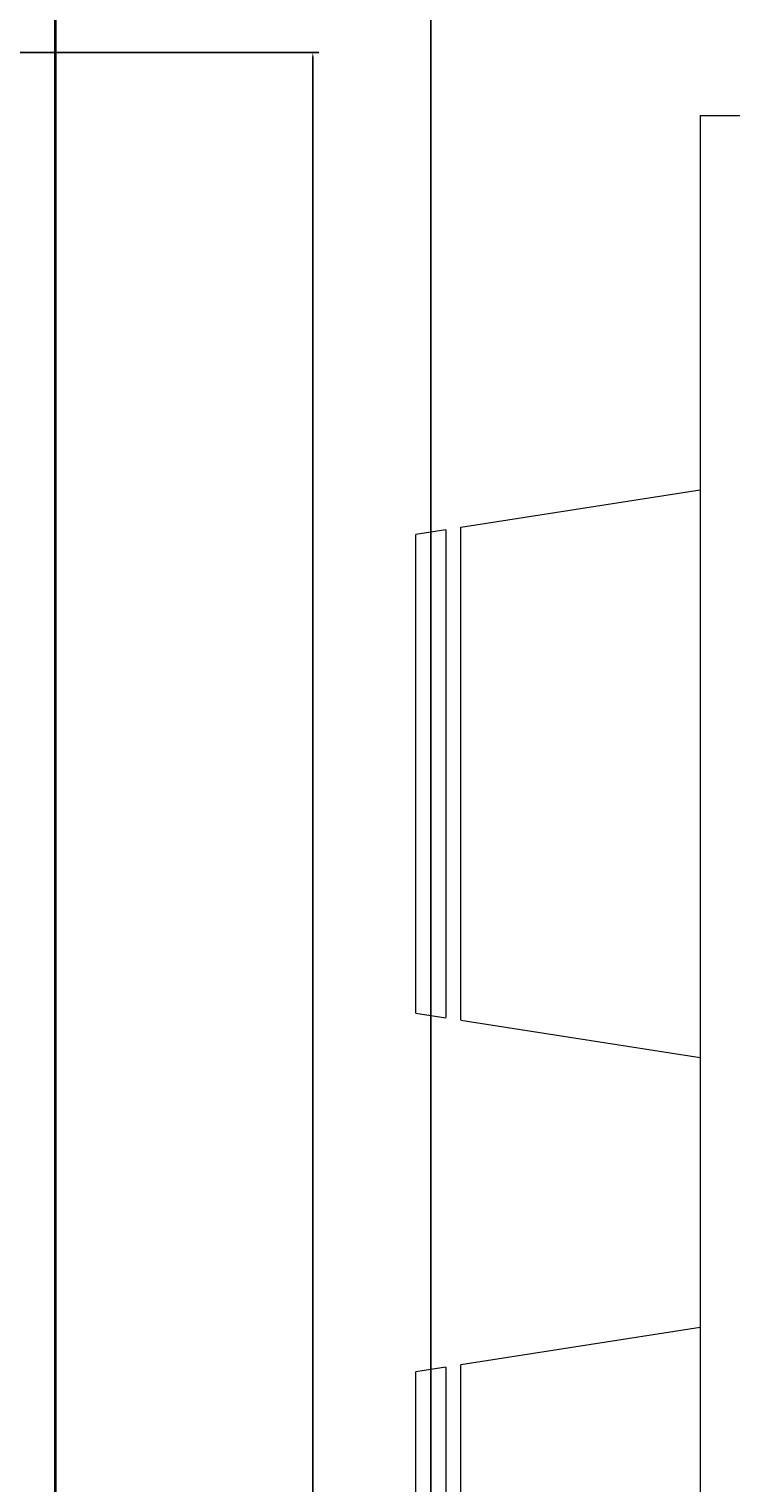
# Model space of a CAD drawing. Units: feet. Extents: x 1654 to 2985, y 1348 to 2230.
# Tile 28 of 53: x 1956 to 1977, y 1820 to 1863. Entities that reach past the tile are written whole.
import ezdxf

# ---------------------------------------------------------------- set-up
doc = ezdxf.new("R2010")
doc.units = ezdxf.units.FT
for name, color, linetype, lineweight in [('A-ANNO-DIMS', 2, 'Continuous', 18), ('A-FURN', 8, 'Continuous', 13), ('A-WALL', 7, 'Continuous', 35)]:
    doc.layers.add(name, color=color, linetype=linetype, lineweight=lineweight)
doc.styles.get("Standard").update_dxf_attribs({"font": 'arial.ttf'})
doc.dimstyles.get("Standard").update_dxf_attribs({"dimtxt": 0.18, "dimasz": 0.18, "dimexe": 0.18, "dimexo": 0.0625, "dimgap": 0.09, "dimtad": 0, "dimtih": 1, "dimtoh": 1, "dimdec": 4, "dimzin": 0, "dimdsep": 46, "dimtxsty": 'Standard', "dimcen": 0.09, "dimadec": 0, "dimazin": 0, "dimtfac": 1, "dimtdec": 4, "dimtofl": 0, "dimtmove": 0, "dimatfit": 3, "dimfxl": 1, "dimtolj": 1, "dimtzin": 0, "dimarcsym": 0})

# ---------------------------------------------------------------- blocks, each defined once
blk = doc.blocks.new('Dining Set - 36 x 72 in.')
for p, q in [((-22, 27.5), (-6, 27.5)), ((-5.8437, 26.49966), (-6, 27.5)), ((6, 27.5), (5.8438, 26.50042)), ((6, 27.5), (22, 27.5)), ((22.1563, 26.49966), (22, 27.5)), ((-5.8416, 26.5), (-22.1534, 26.5)), ((22.1584, 26.5), (5.8466, 26.5)), ((-22.2304, 26), (-5.7608, 26)), ((-4.5152, 17.99762), (-5.7655, 25.99926)), ((5.7657, 26.00059), (4.5153, 17.99762)), ((5.7696, 26), (22.2392, 26)), ((23.4848, 17.99762), (22.2345, 25.99926)), ((36, 18), (-36, 18)), ((36, -18), (36, 18))]:
    blk.add_line(p, q)
blk = doc.blocks.new('*D74')
at = {"layer": 'A-ANNO-DIMS', "color": 0, "lineweight": -2, "transparency": 16777216}
for p, q in [((1948.155, 1862.255), (1964.922, 1862.255)), ((1964.742, 1862.075), (1964.742, 1806.938)), ((1964.742, 1751.435), (1964.742, 1806.572)), ((1948.155, 1751.255), (1964.922, 1751.255))]:
    blk.add_line(p, q, dxfattribs=at)
at = {"layer": 'A-ANNO-DIMS', "color": 0, "transparency": 16777216}
for points in [[(1964.712, 1862.075), (1964.772, 1862.075), (1964.742, 1862.255)], [(1964.712, 1751.435), (1964.772, 1751.435), (1964.742, 1751.255)]]:
    blk.add_solid(points, dxfattribs=at)
at = {"layer": 'Defpoints', "color": 0, "transparency": 16777216}
for p in [(1948.092, 1862.255), (1964.742, 1862.255), (1948.092, 1751.255)]:
    blk.add_point(p, dxfattribs=at)
at = {"layer": 'A-ANNO-DIMS', "color": 0, "transparency": 16777216, "insert": (1964.742, 1806.755), "char_height": 0.18, "attachment_point": 5}
blk.add_mtext('\\A1;COUNTER 111 TYP.', dxfattribs=at)
blk = doc.blocks.new('*D97')
at = {"layer": 'A-ANNO-DIMS', "color": 0, "lineweight": -2, "transparency": 16777216}
for p, q in [((1957.092, 2108.192), (1957.092, 1534.075)), ((1968.254, 2108.192), (1968.254, 1534.075)), ((1957.272, 1534.255), (1962.219, 1534.255)), ((1968.074, 1534.255), (1963.128, 1534.255))]:
    blk.add_line(p, q, dxfattribs=at)
at = {"layer": 'A-ANNO-DIMS', "color": 0, "transparency": 16777216}
for points in [[(1957.272, 1534.285), (1957.272, 1534.225), (1957.092, 1534.255)], [(1968.074, 1534.285), (1968.074, 1534.225), (1968.254, 1534.255)]]:
    blk.add_solid(points, dxfattribs=at)
at = {"layer": 'Defpoints', "color": 0, "transparency": 16777216}
for p in [(1957.092, 2108.255), (1968.254, 2108.255), (1968.254, 1534.255)]:
    blk.add_point(p, dxfattribs=at)
at = {"layer": 'A-ANNO-DIMS', "color": 0, "transparency": 16777216, "insert": (1962.673, 1534.255), "char_height": 0.18, "attachment_point": 5}
blk.add_mtext('\\A1;11.162', dxfattribs=at)

msp = doc.modelspace()

# ---------------------------------------------------------------- linework, layer by layer
at = {"layer": 'A-WALL'}
msp.add_line((1957.0924, 1777.2549), (1957.0924, 1886.2549), dxfattribs=at)

# ---------------------------------------------------------------- block references
at = {"layer": 'A-FURN', "xscale": 0.8893748792417884, "yscale": 0.8893748792417884, "zscale": 0.8893748792417884, "rotation": 90}
msp.add_blockref('Dining Set - 36 x 72 in.', (1992.2681, 1828.3522), dxfattribs=at)

# ---------------------------------------------------------------- dimensions: what is measured, and where the dimension line sits
at = {"layer": 'A-ANNO-DIMS'}
dim = msp.add_linear_dim(base=(1968.2542, 1534.2549), p1=(1957.0924, 2108.2549), p2=(1968.2542, 2108.2549), dimstyle='Standard', override={"dimdec": 3, "dimlfac": 1, "dimrnd": 0, "dimzin": 0, "dimdsep": 46, "dimlunit": 2}, dxfattribs=at)
dim.commit()
dim.dimension.update_dxf_attribs({"geometry": '*D97', "text_midpoint": (1962.6733, 1534.2549)})
dim = msp.add_linear_dim(base=(1964.7424, 1862.2549), p1=(1948.0924, 1751.2549), p2=(1948.0924, 1862.2549), angle=90, text='COUNTER <> TYP.', dimstyle='Standard', override={"dimdec": 0, "dimlfac": 1, "dimrnd": 0, "dimzin": 0, "dimdsep": 46, "dimlunit": 2}, dxfattribs=at)
dim.commit()
dim.dimension.update_dxf_attribs({"geometry": '*D74', "text_midpoint": (1964.7424, 1806.7549)})

doc.saveas('drawing.dxf')
